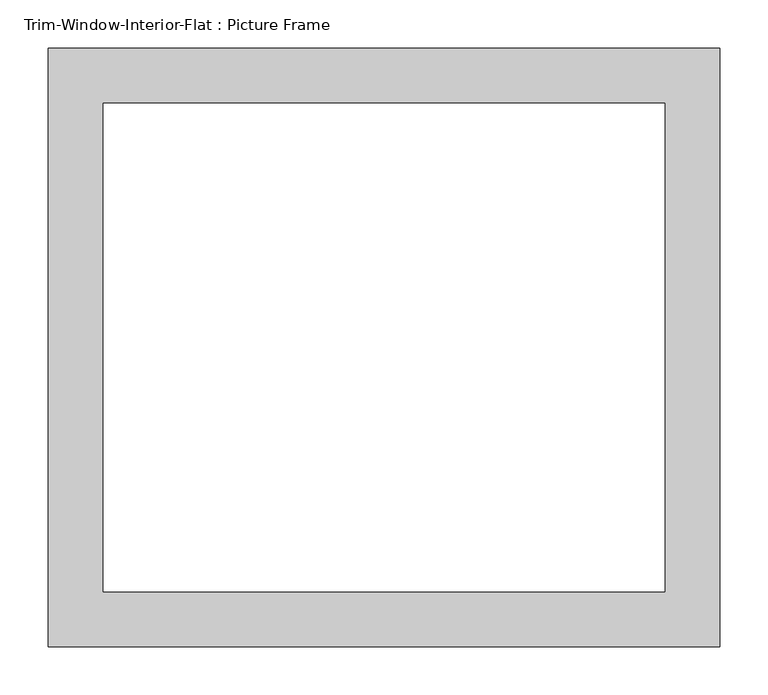
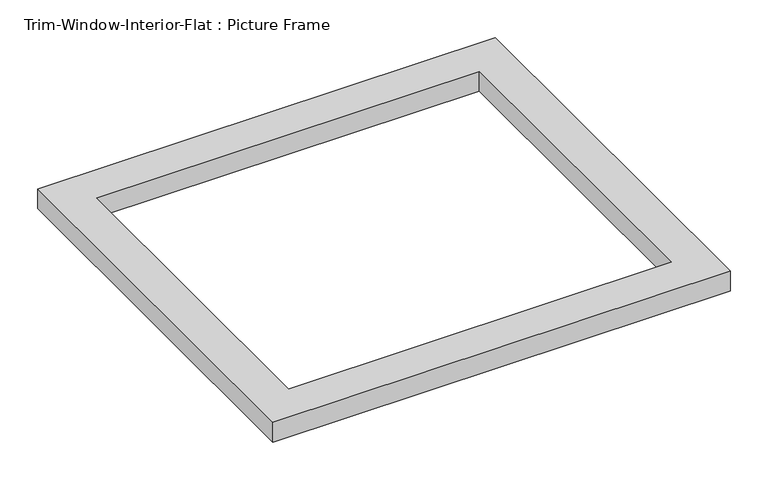
"""IFC4 building model written with IfcOpenShell, lengths in millimetres: proxy geometry, Trim-Window-Interior-Flat : Picture Frame."""

from ifc_helpers import new_model, si_unit, origin, origin_with_axes, place, context, project, spatial, polyline, outline, extrude, source, transform, mapped, element, save


def trim_window_interior_flat_picture_frame_9a74d23d(model_context):
    return source(origin(), model_context, "Body", "SweptSolid", [
        extrude(outline(polyline([(349.25, 44.45), (349.25, -577.85), (-349.25, -577.85), (-349.25, 44.45), (349.25, 44.45)]), holes=[polyline([(292.1, -12.7), (-292.1, -12.7), (-292.1, -520.7), (292.1, -520.7), (292.1, -12.7)])]), origin_with_axes(), (0.0, 0.0, 1.0), 31.75),
    ])


if __name__ == "__main__":
    model = new_model("IFC4")
    model_context = context("Model", 3, world=origin())
    ifc_project = project(units=[si_unit("LENGTHUNIT", "METRE", prefix="MILLI")], contexts=[model_context])
    site = spatial("IfcSite", under=ifc_project)
    building = spatial("IfcBuilding", under=site)
    placement = place(None, origin())
    trim_window_interior_flat_picture_frame_shape = trim_window_interior_flat_picture_frame_9a74d23d(model_context)
    element("IfcBuildingElementProxy", 1, Name="Trim-Window-Interior-Flat : Picture Frame", ObjectType="Trim-Window-Interior-Flat : Picture Frame", at=placement, inside=building, context=model_context, shape_type="MappedRepresentation", body=[
        mapped(trim_window_interior_flat_picture_frame_shape, transform((0.0, 0.0, 0.0), x_axis=(1.0, 0.0, 0.0), y_axis=(0.0, 1.0, 0.0), z_axis=(0.0, 0.0, 1.0))),
    ])
    save(model, "model.ifc")

# Revit data of these elements
# Type "Trim-Window-Interior-Flat : Picture Frame"
#   Trim Thickness_Picture Frame = 0' - 1 1/4"
#   Trim Width = 0' - 2 1/4"
#   Trim Thickness_with Sill = 0' - 0 3/4"
#   Sill Thickness = 0' - 1 1/4"
#   Opening Width [instance default] = 2' - 0"
#   Opening Height [instance default] = 3' - 0"
#   Default Elevation = 4' - 0"
#   Sill = no
#   Picture Frame = yes
#   Trim Material [instance default] = none
# Element 1 (IfcBuildingElementProxy, "Trim-Window-Interior-Flat : Picture Frame")
#   Opening Height = 1' - 9"
#   Trim Material = Wood - Stained
#   Materials on its faces: "Wood - Stained"
# Materials
#   "Wood - Stained": class "Wood", colour RGB 224 178 126, transparency 0, Cost = 0
